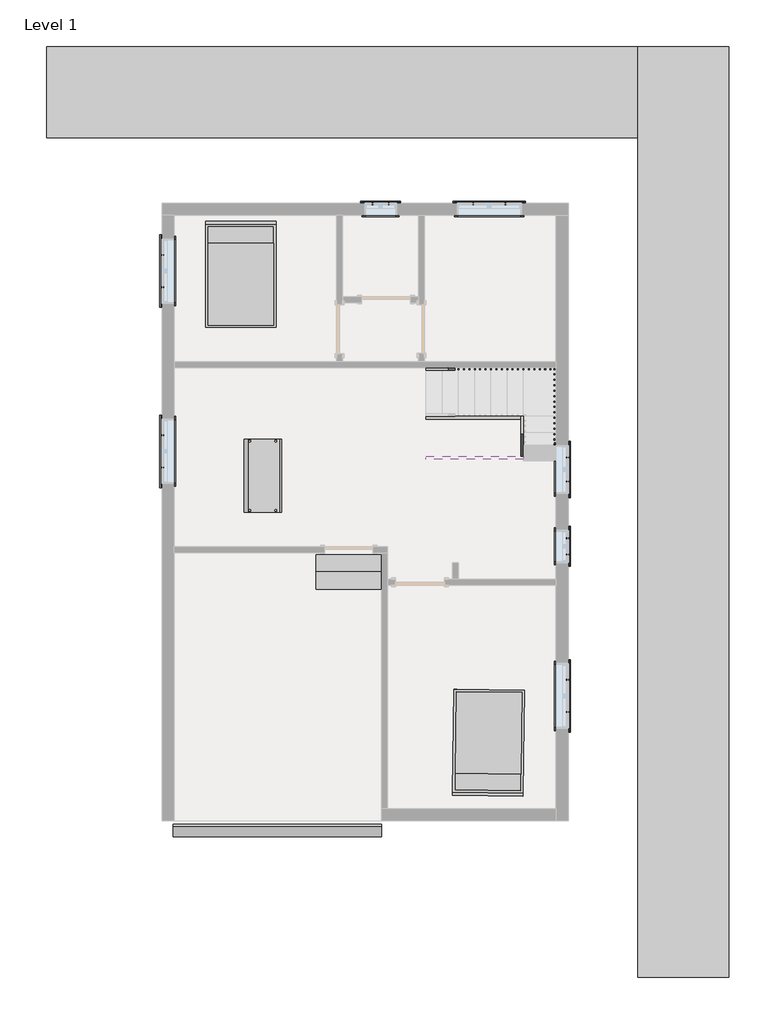
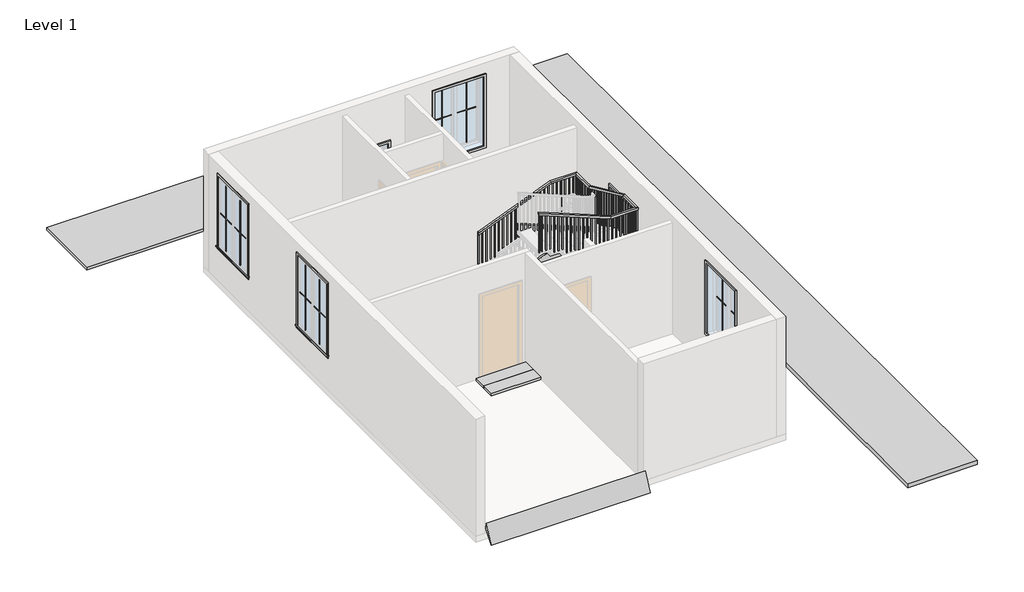
# One storey, part 2 of 2: 33 proxies, 3 members, 2 furniture elements, 1 railing.
"""IFC4 building model written with IfcOpenShell, lengths in millimetres."""

from ifc_helpers import new_model, si_unit, frame, origin, place, context, project, spatial, polyline, outline, extrude, faceted_brep, transform, mapped, element, save
from components import extrusion_extrusion_7330b34c, generic_models_1_generic_models_1_3256bdb4, generic_models_2_generic_models_2_0ca87cec, generic_models_3_generic_models_3_c0206aab, modern_coffee_table_17989_modern_coffee_table_17989_d3a860c8, muntin_pattern_2x2_muntin_pattern_2x2_2b4d9f72, muntin_pattern_2x2_muntin_pattern_2x2_ef995ed3, muntin_pattern_2x2_muntin_pattern_2x2_53152e2c, muntin_pattern_2x2_muntin_pattern_2x2_e8f3e573, muntin_pattern_2x2_muntin_pattern_2x2_9b64c8d5, muntin_pattern_2x2_muntin_pattern_2x2_d319fd2e, trim_window_exterior_flat_with_sill_b7e4d11c, trim_window_exterior_flat_with_sill_a665a915, trim_window_exterior_flat_with_sill_66148908, trim_window_interior_flat_picture_frame_936b8d2a, trim_window_interior_flat_picture_frame_d485c387, trim_window_interior_flat_picture_frame_d5b7f3a4, bed_17739_bed_17739_15c61121

model = new_model("IFC4")

# Units and contexts
model_context = context("Model", 3, world=origin())
ifc_project = project(units=[si_unit("LENGTHUNIT", "METRE", prefix="MILLI")], contexts=[model_context])

# Site, building, storey
site = spatial("IfcSite", under=ifc_project)
building = spatial("IfcBuilding", under=site)
storey = spatial("IfcBuildingStorey", under=building, Name="Level 1", Elevation=0.0)

# Proxies
placement = place(None, origin())
extrusion_extrusion_shape = extrusion_extrusion_7330b34c(model_context)
element("IfcBuildingElementProxy", 1, Name="EXTRUSION : EXTRUSION", ObjectType="EXTRUSION : EXTRUSION", at=placement, inside=storey, context=model_context, shape_type="MappedRepresentation", body=[
    mapped(extrusion_extrusion_shape, transform((0.0, 0.0, 0.0), x_axis=(1.0, 0.0, 0.0), y_axis=(0.0, 1.0, 0.0), z_axis=(0.0, 0.0, 1.0))),
])
generic_models_1_generic_models_1_shape = generic_models_1_generic_models_1_3256bdb4(model_context)
element("IfcBuildingElementProxy", 2, Name="Generic Models 1 : Generic Models 1", ObjectType="Generic Models 1 : Generic Models 1", at=placement, inside=storey, context=model_context, shape_type="MappedRepresentation", body=[
    mapped(generic_models_1_generic_models_1_shape, transform((0.0, 0.0, 0.0), x_axis=(1.0, 0.0, 0.0), y_axis=(0.0, 1.0, 0.0), z_axis=(0.0, 0.0, 1.0))),
])
generic_models_2_generic_models_2_shape = generic_models_2_generic_models_2_0ca87cec(model_context)
element("IfcBuildingElementProxy", 3, Name="Generic Models 2 : Generic Models 2", ObjectType="Generic Models 2 : Generic Models 2", at=placement, inside=storey, context=model_context, shape_type="MappedRepresentation", body=[
    mapped(generic_models_2_generic_models_2_shape, transform((0.0, 0.0, 0.0), x_axis=(1.0, 0.0, 0.0), y_axis=(0.0, 1.0, 0.0), z_axis=(0.0, 0.0, 1.0))),
])
generic_models_3_generic_models_3_shape = generic_models_3_generic_models_3_c0206aab(model_context)
element("IfcBuildingElementProxy", 4, Name="Generic Models 3 : Generic Models 3", ObjectType="Generic Models 3 : Generic Models 3", at=placement, inside=storey, context=model_context, shape_type="MappedRepresentation", body=[
    mapped(generic_models_3_generic_models_3_shape, transform((0.0, 0.0, 0.0), x_axis=(1.0, 0.0, 0.0), y_axis=(0.0, 1.0, 0.0), z_axis=(0.0, 0.0, 1.0))),
])
modern_coffee_table_17989_modern_coffee_table_17989_shape = modern_coffee_table_17989_modern_coffee_table_17989_d3a860c8(model_context)
element("IfcBuildingElementProxy", 5, Name="Modern_Coffee_Table_17989 : Modern_Coffee_Table_17989", ObjectType="Modern_Coffee_Table_17989 : Modern_Coffee_Table_17989", at=placement, inside=storey, context=model_context, shape_type="MappedRepresentation", body=[
    mapped(modern_coffee_table_17989_modern_coffee_table_17989_shape, transform((3060.7, 9172.1823212, 0.0), x_axis=(0.0, 1.0, 0.0), y_axis=(-1.0, 0.0, 0.0), z_axis=(0.0, 0.0, 1.0))),
])
muntin_pattern_2x2_muntin_pattern_2x2_shape = muntin_pattern_2x2_muntin_pattern_2x2_2b4d9f72(model_context)
element("IfcBuildingElementProxy", 6, Name="Muntin Pattern_2x2 : Muntin Pattern_2x2", ObjectType="Muntin Pattern_2x2 : Muntin Pattern_2x2", at=placement, inside=storey, context=model_context, shape_type="MappedRepresentation", body=[
    mapped(muntin_pattern_2x2_muntin_pattern_2x2_shape, transform((1533.525, 12477.4069306, 984.25), x_axis=(0.0, 1.0, 0.0), y_axis=(-1.0, 0.0, 0.0), z_axis=(0.0, 0.0, 1.0))),
])
element("IfcBuildingElementProxy", 7, Name="Muntin Pattern_2x2 : Muntin Pattern_2x2", ObjectType="Muntin Pattern_2x2 : Muntin Pattern_2x2", at=placement, inside=storey, context=model_context, shape_type="MappedRepresentation", body=[
    mapped(muntin_pattern_2x2_muntin_pattern_2x2_shape, transform((7361.2375, 14045.8073212, 984.25), x_axis=(1.0, 0.0, 0.0), y_axis=(0.0, 1.0, 0.0), z_axis=(0.0, 0.0, 1.0))),
])
element("IfcBuildingElementProxy", 8, Name="Muntin Pattern_2x2 : Muntin Pattern_2x2", ObjectType="Muntin Pattern_2x2 : Muntin Pattern_2x2", at=placement, inside=storey, context=model_context, shape_type="MappedRepresentation", body=[
    mapped(muntin_pattern_2x2_muntin_pattern_2x2_shape, transform((9134.475, 5119.2948212, 984.25), x_axis=(0.0, -1.0, 0.0), y_axis=(1.0, 0.0, 0.0), z_axis=(0.0, 0.0, 1.0))),
])
element("IfcBuildingElementProxy", 9, Name="Muntin Pattern_2x2 : Muntin Pattern_2x2", ObjectType="Muntin Pattern_2x2 : Muntin Pattern_2x2", at=placement, inside=storey, context=model_context, shape_type="MappedRepresentation", body=[
    mapped(muntin_pattern_2x2_muntin_pattern_2x2_shape, transform((1533.525, 9097.5698212, 984.25), x_axis=(0.0, 1.0, 0.0), y_axis=(-1.0, 0.0, 0.0), z_axis=(0.0, 0.0, 1.0))),
])
muntin_pattern_2x2_muntin_pattern_2x2_2_shape = muntin_pattern_2x2_muntin_pattern_2x2_ef995ed3(model_context)
element("IfcBuildingElementProxy", 10, Name="Muntin Pattern_2x2 : Muntin Pattern_2x2", ObjectType="Muntin Pattern_2x2 : Muntin Pattern_2x2", at=placement, inside=storey, context=model_context, shape_type="MappedRepresentation", body=[
    mapped(muntin_pattern_2x2_muntin_pattern_2x2_2_shape, transform((1533.525, 13083.8319306, 984.25), x_axis=(0.0, -1.0, 0.0), y_axis=(1.0, 0.0, 0.0), z_axis=(0.0, 0.0, 1.0))),
])
element("IfcBuildingElementProxy", 11, Name="Muntin Pattern_2x2 : Muntin Pattern_2x2", ObjectType="Muntin Pattern_2x2 : Muntin Pattern_2x2", at=placement, inside=storey, context=model_context, shape_type="MappedRepresentation", body=[
    mapped(muntin_pattern_2x2_muntin_pattern_2x2_2_shape, transform((7967.6625, 14045.8073212, 984.25), x_axis=(-1.0, 0.0, 0.0), y_axis=(0.0, -1.0, 0.0), z_axis=(0.0, 0.0, 1.0))),
])
element("IfcBuildingElementProxy", 12, Name="Muntin Pattern_2x2 : Muntin Pattern_2x2", ObjectType="Muntin Pattern_2x2 : Muntin Pattern_2x2", at=placement, inside=storey, context=model_context, shape_type="MappedRepresentation", body=[
    mapped(muntin_pattern_2x2_muntin_pattern_2x2_2_shape, transform((9134.475, 4512.8698212, 984.25), x_axis=(0.0, 1.0, 0.0), y_axis=(-1.0, 0.0, 0.0), z_axis=(0.0, 0.0, 1.0))),
])
element("IfcBuildingElementProxy", 13, Name="Muntin Pattern_2x2 : Muntin Pattern_2x2", ObjectType="Muntin Pattern_2x2 : Muntin Pattern_2x2", at=placement, inside=storey, context=model_context, shape_type="MappedRepresentation", body=[
    mapped(muntin_pattern_2x2_muntin_pattern_2x2_2_shape, transform((1533.525, 9703.9948212, 984.25), x_axis=(0.0, -1.0, 0.0), y_axis=(1.0, 0.0, 0.0), z_axis=(0.0, 0.0, 1.0))),
])
muntin_pattern_2x2_muntin_pattern_2x2_3_shape = muntin_pattern_2x2_muntin_pattern_2x2_53152e2c(model_context)
element("IfcBuildingElementProxy", 14, Name="Muntin Pattern_2x2 : Muntin Pattern_2x2", ObjectType="Muntin Pattern_2x2 : Muntin Pattern_2x2", at=placement, inside=storey, context=model_context, shape_type="MappedRepresentation", body=[
    mapped(muntin_pattern_2x2_muntin_pattern_2x2_3_shape, transform((9134.475, 7771.2135712, 984.25), x_axis=(0.0, -1.0, 0.0), y_axis=(1.0, 0.0, 0.0), z_axis=(0.0, 0.0, 1.0))),
])
element("IfcBuildingElementProxy", 15, Name="Muntin Pattern_2x2 : Muntin Pattern_2x2", ObjectType="Muntin Pattern_2x2 : Muntin Pattern_2x2", at=placement, inside=storey, context=model_context, shape_type="MappedRepresentation", body=[
    mapped(muntin_pattern_2x2_muntin_pattern_2x2_3_shape, transform((5475.2875, 14045.8073212, 984.25), x_axis=(1.0, 0.0, 0.0), y_axis=(0.0, 1.0, 0.0), z_axis=(0.0, 0.0, 1.0))),
])
muntin_pattern_2x2_muntin_pattern_2x2_4_shape = muntin_pattern_2x2_muntin_pattern_2x2_e8f3e573(model_context)
element("IfcBuildingElementProxy", 16, Name="Muntin Pattern_2x2 : Muntin Pattern_2x2", ObjectType="Muntin Pattern_2x2 : Muntin Pattern_2x2", at=placement, inside=storey, context=model_context, shape_type="MappedRepresentation", body=[
    mapped(muntin_pattern_2x2_muntin_pattern_2x2_4_shape, transform((9134.475, 7469.5885712, 984.25), x_axis=(0.0, 1.0, 0.0), y_axis=(-1.0, 0.0, 0.0), z_axis=(0.0, 0.0, 1.0))),
])
element("IfcBuildingElementProxy", 17, Name="Muntin Pattern_2x2 : Muntin Pattern_2x2", ObjectType="Muntin Pattern_2x2 : Muntin Pattern_2x2", at=placement, inside=storey, context=model_context, shape_type="MappedRepresentation", body=[
    mapped(muntin_pattern_2x2_muntin_pattern_2x2_4_shape, transform((5776.9125, 14045.8073212, 984.25), x_axis=(-1.0, 0.0, 0.0), y_axis=(0.0, -1.0, 0.0), z_axis=(0.0, 0.0, 1.0))),
])
muntin_pattern_2x2_muntin_pattern_2x2_5_shape = muntin_pattern_2x2_muntin_pattern_2x2_9b64c8d5(model_context)
element("IfcBuildingElementProxy", 18, Name="Muntin Pattern_2x2 : Muntin Pattern_2x2", ObjectType="Muntin Pattern_2x2 : Muntin Pattern_2x2", at=placement, inside=storey, context=model_context, shape_type="MappedRepresentation", body=[
    mapped(muntin_pattern_2x2_muntin_pattern_2x2_5_shape, transform((9134.475, 9287.1024384, 984.25), x_axis=(0.0, -1.0, 0.0), y_axis=(1.0, 0.0, 0.0), z_axis=(0.0, 0.0, 1.0))),
])
muntin_pattern_2x2_muntin_pattern_2x2_6_shape = muntin_pattern_2x2_muntin_pattern_2x2_d319fd2e(model_context)
element("IfcBuildingElementProxy", 19, Name="Muntin Pattern_2x2 : Muntin Pattern_2x2", ObjectType="Muntin Pattern_2x2 : Muntin Pattern_2x2", at=placement, inside=storey, context=model_context, shape_type="MappedRepresentation", body=[
    mapped(muntin_pattern_2x2_muntin_pattern_2x2_6_shape, transform((9134.475, 8833.0774384, 984.25), x_axis=(0.0, 1.0, 0.0), y_axis=(-1.0, 0.0, 0.0), z_axis=(0.0, 0.0, 1.0))),
])
trim_window_exterior_flat_with_sill_shape = trim_window_exterior_flat_with_sill_b7e4d11c(model_context)
element("IfcBuildingElementProxy", 20, Name="Trim-Window-Exterior-Flat : with Sill", ObjectType="Trim-Window-Exterior-Flat : with Sill", at=placement, inside=storey, context=model_context, shape_type="MappedRepresentation", body=[
    mapped(trim_window_exterior_flat_with_sill_shape, transform((1524.0, 12780.6194306, 2743.2), x_axis=(0.0, -1.0, 0.0), y_axis=(0.0, 0.0, 1.0), z_axis=(-1.0, 0.0, 0.0))),
])
element("IfcBuildingElementProxy", 21, Name="Trim-Window-Exterior-Flat : with Sill", ObjectType="Trim-Window-Exterior-Flat : with Sill", at=placement, inside=storey, context=model_context, shape_type="MappedRepresentation", body=[
    mapped(trim_window_exterior_flat_with_sill_shape, transform((7664.45, 14055.3323212, 2743.2), x_axis=(-1.0, 0.0, 0.0), y_axis=(0.0, 0.0, 1.0), z_axis=(0.0, 1.0, 0.0))),
])
element("IfcBuildingElementProxy", 22, Name="Trim-Window-Exterior-Flat : with Sill", ObjectType="Trim-Window-Exterior-Flat : with Sill", at=placement, inside=storey, context=model_context, shape_type="MappedRepresentation", body=[
    mapped(trim_window_exterior_flat_with_sill_shape, transform((9144.0, 4816.0823212, 2743.2), x_axis=(0.0, 1.0, 0.0), y_axis=(0.0, 0.0, 1.0), z_axis=(1.0, 0.0, 0.0))),
])
element("IfcBuildingElementProxy", 23, Name="Trim-Window-Exterior-Flat : with Sill", ObjectType="Trim-Window-Exterior-Flat : with Sill", at=placement, inside=storey, context=model_context, shape_type="MappedRepresentation", body=[
    mapped(trim_window_exterior_flat_with_sill_shape, transform((1524.0, 9400.7823212, 2743.2), x_axis=(0.0, -1.0, 0.0), y_axis=(0.0, 0.0, 1.0), z_axis=(-1.0, 0.0, 0.0))),
])
trim_window_exterior_flat_with_sill_2_shape = trim_window_exterior_flat_with_sill_a665a915(model_context)
element("IfcBuildingElementProxy", 24, Name="Trim-Window-Exterior-Flat : with Sill", ObjectType="Trim-Window-Exterior-Flat : with Sill", at=placement, inside=storey, context=model_context, shape_type="MappedRepresentation", body=[
    mapped(trim_window_exterior_flat_with_sill_2_shape, transform((9144.0, 7620.4010712, 1828.8), x_axis=(0.0, 1.0, 0.0), y_axis=(0.0, 0.0, 1.0), z_axis=(1.0, 0.0, 0.0))),
])
element("IfcBuildingElementProxy", 25, Name="Trim-Window-Exterior-Flat : with Sill", ObjectType="Trim-Window-Exterior-Flat : with Sill", at=placement, inside=storey, context=model_context, shape_type="MappedRepresentation", body=[
    mapped(trim_window_exterior_flat_with_sill_2_shape, transform((5626.1, 14055.3323212, 1828.8), x_axis=(-1.0, 0.0, 0.0), y_axis=(0.0, 0.0, 1.0), z_axis=(0.0, 1.0, 0.0))),
])
trim_window_exterior_flat_with_sill_3_shape = trim_window_exterior_flat_with_sill_66148908(model_context)
element("IfcBuildingElementProxy", 26, Name="Trim-Window-Exterior-Flat : with Sill", ObjectType="Trim-Window-Exterior-Flat : with Sill", at=placement, inside=storey, context=model_context, shape_type="MappedRepresentation", body=[
    mapped(trim_window_exterior_flat_with_sill_3_shape, transform((9144.0, 9060.0899384, 2260.6), x_axis=(0.0, 1.0, 0.0), y_axis=(0.0, 0.0, 1.0), z_axis=(1.0, 0.0, 0.0))),
])
trim_window_interior_flat_picture_frame_shape = trim_window_interior_flat_picture_frame_936b8d2a(model_context)
element("IfcBuildingElementProxy", 27, Name="Trim-Window-Interior-Flat : Picture Frame", ObjectType="Trim-Window-Interior-Flat : Picture Frame", at=placement, inside=storey, context=model_context, shape_type="MappedRepresentation", body=[
    mapped(trim_window_interior_flat_picture_frame_shape, transform((1752.6, 12780.6194306, 2743.2), x_axis=(0.0, 1.0, 0.0), y_axis=(0.0, 0.0, 1.0), z_axis=(1.0, 0.0, 0.0))),
])
element("IfcBuildingElementProxy", 28, Name="Trim-Window-Interior-Flat : Picture Frame", ObjectType="Trim-Window-Interior-Flat : Picture Frame", at=placement, inside=storey, context=model_context, shape_type="MappedRepresentation", body=[
    mapped(trim_window_interior_flat_picture_frame_shape, transform((7664.45, 13826.7323212, 2743.2), x_axis=(1.0, 0.0, 0.0), y_axis=(0.0, 0.0, 1.0), z_axis=(0.0, -1.0, 0.0))),
])
element("IfcBuildingElementProxy", 29, Name="Trim-Window-Interior-Flat : Picture Frame", ObjectType="Trim-Window-Interior-Flat : Picture Frame", at=placement, inside=storey, context=model_context, shape_type="MappedRepresentation", body=[
    mapped(trim_window_interior_flat_picture_frame_shape, transform((8915.4, 4816.0823212, 2743.2), x_axis=(0.0, -1.0, 0.0), y_axis=(0.0, 0.0, 1.0), z_axis=(-1.0, 0.0, 0.0))),
])
element("IfcBuildingElementProxy", 30, Name="Trim-Window-Interior-Flat : Picture Frame", ObjectType="Trim-Window-Interior-Flat : Picture Frame", at=placement, inside=storey, context=model_context, shape_type="MappedRepresentation", body=[
    mapped(trim_window_interior_flat_picture_frame_shape, transform((1752.6, 9400.7823212, 2743.2), x_axis=(0.0, 1.0, 0.0), y_axis=(0.0, 0.0, 1.0), z_axis=(1.0, 0.0, 0.0))),
])
trim_window_interior_flat_picture_frame_2_shape = trim_window_interior_flat_picture_frame_d485c387(model_context)
element("IfcBuildingElementProxy", 31, Name="Trim-Window-Interior-Flat : Picture Frame", ObjectType="Trim-Window-Interior-Flat : Picture Frame", at=placement, inside=storey, context=model_context, shape_type="MappedRepresentation", body=[
    mapped(trim_window_interior_flat_picture_frame_2_shape, transform((8915.4, 7620.4010712, 1828.8), x_axis=(0.0, -1.0, 0.0), y_axis=(0.0, 0.0, 1.0), z_axis=(-1.0, 0.0, 0.0))),
])
element("IfcBuildingElementProxy", 32, Name="Trim-Window-Interior-Flat : Picture Frame", ObjectType="Trim-Window-Interior-Flat : Picture Frame", at=placement, inside=storey, context=model_context, shape_type="MappedRepresentation", body=[
    mapped(trim_window_interior_flat_picture_frame_2_shape, transform((5626.1, 13826.7323212, 1828.8), x_axis=(1.0, 0.0, 0.0), y_axis=(0.0, 0.0, 1.0), z_axis=(0.0, -1.0, 0.0))),
])
trim_window_interior_flat_picture_frame_3_shape = trim_window_interior_flat_picture_frame_d5b7f3a4(model_context)
element("IfcBuildingElementProxy", 33, Name="Trim-Window-Interior-Flat : Picture Frame", ObjectType="Trim-Window-Interior-Flat : Picture Frame", at=placement, inside=storey, context=model_context, shape_type="MappedRepresentation", body=[
    mapped(trim_window_interior_flat_picture_frame_3_shape, transform((8915.4, 9060.0899384, 2260.6), x_axis=(0.0, -1.0, 0.0), y_axis=(0.0, 0.0, 1.0), z_axis=(-1.0, 0.0, 0.0))),
])

# Furniture
bed_17739_bed_17739_shape = bed_17739_bed_17739_15c61121(model_context)
element("IfcFurniture", 34, ObjectType="Bed_17739 : Bed_17739", at=placement, inside=storey, context=model_context, shape_type="MappedRepresentation", body=[
    mapped(bed_17739_bed_17739_shape, transform((3003.55, 12696.4323212, 0.0), x_axis=(1.0, 0.0, 0.0), y_axis=(0.0, 1.0, 0.0), z_axis=(0.0, 0.0, 1.0))),
])
element("IfcFurniture", 35, ObjectType="Bed_17739 : Bed_17739", at=placement, inside=storey, context=model_context, shape_type="MappedRepresentation", body=[
    mapped(bed_17739_bed_17739_shape, transform((7650.1504891, 3963.5673274, 0.0), x_axis=(-0.9999063358908578, 0.013686469424921632, 0.0), y_axis=(-0.013686469424921632, -0.9999063358908578, 0.0), z_axis=(0.0, 0.0, 1.0))),
])

# Members
element("IfcMember", 36, ObjectType="Stringer - 2\" Width", at=placement, inside=storey, context=model_context, shape_type="SweptSolid", body=[
    extrude(outline(polyline([(196.3880536, 6477.0), (0.0, 6477.0), (0.0, 6806.7289826), (579.3084069, 8255.0), (907.5880536, 8255.0), (196.3880536, 6477.0)])), frame((0.0, 10004.0323212, 0.0), z_axis=(0.0, 1.0, 0.0), x_axis=(0.0, 0.0, 1.0)), (0.0, 0.0, 1.0), 50.8),
])
element("IfcMember", 37, ObjectType="Stringer - 2\" Width", at=placement, inside=storey, context=model_context, shape_type="SweptSolid", body=[
    extrude(outline(polyline([(10054.8323212, 1053.4437705), (10054.8323212, 718.3051732), (9305.5323212, 1060.842316), (9305.5323212, 1395.9809133), (10054.8323212, 1053.4437705)])), frame((8255.0, 0.0, 0.0), z_axis=(1.0, 0.0, 0.0), x_axis=(0.0, 1.0, 0.0)), (0.0, 0.0, 1.0), 50.8),
])
element("IfcMember", 38, ObjectType="Stringer - 2\" Width", at=placement, inside=storey, context=model_context, shape_type="SweptSolid", body=[
    extrude(outline(polyline([(1209.2284069, 8305.8), (1537.5080536, 8305.8), (2269.0280536, 6477.0), (1940.7484069, 6477.0), (1209.2284069, 8305.8)])), frame((0.0, 9254.7323212, 0.0), z_axis=(0.0, 1.0, 0.0), x_axis=(0.0, 0.0, 1.0)), (0.0, 0.0, 1.0), 50.8),
])

# Railing
element("IfcRailing", 39, ObjectType="Handrail - Rectangular", at=placement, inside=storey, context=model_context, shape_type="SolidModel", body=[
    faceted_brep([(6477.0, 10969.2323212, 1036.32), (6477.0, 10969.2323212, 981.6067256), (6477.0, 10918.4323212, 981.6067256), (6477.0, 10918.4323212, 1036.32), (8242.3, 10969.2323212, 1742.44), (8252.0831861, 10969.2323212, 1691.64), (8252.0831861, 10918.4323212, 1691.64), (8242.3, 10918.4323212, 1742.44), (8915.4, 10969.2323212, 1742.44), (8915.4, 10969.2323212, 1691.64), (8864.6, 10918.4323212, 1691.64), (8864.6, 10918.4323212, 1742.44), (8915.4, 10377.0948212, 1742.44), (8915.4, 10366.0338743, 1691.64), (8864.6, 10366.0338743, 1691.64), (8864.6, 10377.0948212, 1742.44), (8915.4, 8932.4698212, 2402.84), (8915.4, 8921.4088743, 2352.04), (8864.6, 8921.4088743, 2352.04), (8864.6, 8932.4698212, 2402.84), (8915.4, 8340.3323212, 2402.84), (8915.4, 8340.3323212, 2352.04), (8864.6, 8391.1323212, 2352.04), (8864.6, 8391.1323212, 2402.84), (8242.3, 8340.3323212, 2402.84), (8232.5168139, 8340.3323212, 2352.04), (8232.5168139, 8391.1323212, 2352.04), (8242.3, 8391.1323212, 2402.84), (6477.0, 8340.3323212, 3108.96), (6477.0, 8391.1323212, 3108.96), (6477.0, 8391.1323212, 3054.2467256), (6477.0, 8340.3323212, 3054.2467256)], [[[0, 1, 2, 3]], [[1, 0, 4, 5]], [[2, 1, 5, 6]], [[3, 2, 6, 7]], [[0, 3, 7, 4]], [[5, 4, 8, 9]], [[6, 5, 9, 10]], [[7, 6, 10, 11]], [[4, 7, 11, 8]], [[9, 8, 12, 13]], [[10, 9, 13, 14]], [[11, 10, 14, 15]], [[8, 11, 15, 12]], [[13, 12, 16, 17]], [[14, 13, 17, 18]], [[15, 14, 18, 19]], [[12, 15, 19, 16]], [[17, 16, 20, 21]], [[18, 17, 21, 22]], [[19, 18, 22, 23]], [[16, 19, 23, 20]], [[21, 20, 24, 25]], [[22, 21, 25, 26]], [[23, 22, 26, 27]], [[20, 23, 27, 24]], [[28, 29, 30, 31]], [[25, 24, 28, 31]], [[26, 25, 31, 30]], [[27, 26, 30, 29]], [[24, 27, 29, 28]]]),
    extrude(outline(polyline([(3027.5767256, 6543.675), (2072.64, 6543.675), (2072.64, 6562.725), (3019.9567256, 6562.725), (3027.5767256, 6543.675)])), frame((0.0, 8356.2073212, 0.0), z_axis=(0.0, 1.0, 0.0), x_axis=(0.0, 0.0, 1.0)), (0.0, 0.0, 1.0), 19.05),
    extrude(outline(polyline([(2986.9367256, 6645.275), (2072.64, 6645.275), (2072.64, 6664.325), (2979.3167256, 6664.325), (2986.9367256, 6645.275)])), frame((0.0, 8356.2073212, 0.0), z_axis=(0.0, 1.0, 0.0), x_axis=(0.0, 0.0, 1.0)), (0.0, 0.0, 1.0), 19.05),
    extrude(outline(polyline([(2946.2967256, 6746.875), (2072.64, 6746.875), (2072.64, 6765.925), (2938.6767256, 6765.925), (2946.2967256, 6746.875)])), frame((0.0, 8356.2073212, 0.0), z_axis=(0.0, 1.0, 0.0), x_axis=(0.0, 0.0, 1.0)), (0.0, 0.0, 1.0), 19.05),
    extrude(outline(polyline([(2905.6567256, 6848.475), (1950.72, 6848.475), (1950.72, 6867.525), (2898.0367256, 6867.525), (2905.6567256, 6848.475)])), frame((0.0, 8356.2073212, 0.0), z_axis=(0.0, 1.0, 0.0), x_axis=(0.0, 0.0, 1.0)), (0.0, 0.0, 1.0), 19.05),
    extrude(outline(polyline([(2865.0167256, 6950.075), (1950.72, 6950.075), (1950.72, 6969.125), (2857.3967256, 6969.125), (2865.0167256, 6950.075)])), frame((0.0, 8356.2073212, 0.0), z_axis=(0.0, 1.0, 0.0), x_axis=(0.0, 0.0, 1.0)), (0.0, 0.0, 1.0), 19.05),
    extrude(outline(polyline([(2824.3767256, 7051.675), (1950.72, 7051.675), (1950.72, 7070.725), (2816.7567256, 7070.725), (2824.3767256, 7051.675)])), frame((0.0, 8356.2073212, 0.0), z_axis=(0.0, 1.0, 0.0), x_axis=(0.0, 0.0, 1.0)), (0.0, 0.0, 1.0), 19.05),
    extrude(outline(polyline([(2783.7367256, 7153.275), (1828.8, 7153.275), (1828.8, 7172.325), (2776.1167256, 7172.325), (2783.7367256, 7153.275)])), frame((0.0, 8356.2073212, 0.0), z_axis=(0.0, 1.0, 0.0), x_axis=(0.0, 0.0, 1.0)), (0.0, 0.0, 1.0), 19.05),
    extrude(outline(polyline([(2743.0967256, 7254.875), (1828.8, 7254.875), (1828.8, 7273.925), (2735.4767256, 7273.925), (2743.0967256, 7254.875)])), frame((0.0, 8356.2073212, 0.0), z_axis=(0.0, 1.0, 0.0), x_axis=(0.0, 0.0, 1.0)), (0.0, 0.0, 1.0), 19.05),
    extrude(outline(polyline([(2702.4567256, 7356.475), (1828.8, 7356.475), (1828.8, 7375.525), (2694.8367256, 7375.525), (2702.4567256, 7356.475)])), frame((0.0, 8356.2073212, 0.0), z_axis=(0.0, 1.0, 0.0), x_axis=(0.0, 0.0, 1.0)), (0.0, 0.0, 1.0), 19.05),
    extrude(outline(polyline([(2661.8167256, 7458.075), (1706.88, 7458.075), (1706.88, 7477.125), (2654.1967256, 7477.125), (2661.8167256, 7458.075)])), frame((0.0, 8356.2073212, 0.0), z_axis=(0.0, 1.0, 0.0), x_axis=(0.0, 0.0, 1.0)), (0.0, 0.0, 1.0), 19.05),
    extrude(outline(polyline([(2621.1767256, 7559.675), (1706.88, 7559.675), (1706.88, 7578.725), (2613.5567256, 7578.725), (2621.1767256, 7559.675)])), frame((0.0, 8356.2073212, 0.0), z_axis=(0.0, 1.0, 0.0), x_axis=(0.0, 0.0, 1.0)), (0.0, 0.0, 1.0), 19.05),
    extrude(outline(polyline([(2580.5367256, 7661.275), (1706.88, 7661.275), (1706.88, 7680.325), (2572.9167256, 7680.325), (2580.5367256, 7661.275)])), frame((0.0, 8356.2073212, 0.0), z_axis=(0.0, 1.0, 0.0), x_axis=(0.0, 0.0, 1.0)), (0.0, 0.0, 1.0), 19.05),
    extrude(outline(polyline([(2539.8967256, 7762.875), (1584.96, 7762.875), (1584.96, 7781.925), (2532.2767256, 7781.925), (2539.8967256, 7762.875)])), frame((0.0, 8356.2073212, 0.0), z_axis=(0.0, 1.0, 0.0), x_axis=(0.0, 0.0, 1.0)), (0.0, 0.0, 1.0), 19.05),
    extrude(outline(polyline([(2499.2567256, 7864.475), (1584.96, 7864.475), (1584.96, 7883.525), (2491.6367256, 7883.525), (2499.2567256, 7864.475)])), frame((0.0, 8356.2073212, 0.0), z_axis=(0.0, 1.0, 0.0), x_axis=(0.0, 0.0, 1.0)), (0.0, 0.0, 1.0), 19.05),
    extrude(outline(polyline([(2458.6167256, 7966.075), (1584.96, 7966.075), (1584.96, 7985.125), (2450.9967256, 7985.125), (2458.6167256, 7966.075)])), frame((0.0, 8356.2073212, 0.0), z_axis=(0.0, 1.0, 0.0), x_axis=(0.0, 0.0, 1.0)), (0.0, 0.0, 1.0), 19.05),
    extrude(outline(polyline([(2417.9767256, 8067.675), (1463.04, 8067.675), (1463.04, 8086.725), (2410.3567256, 8086.725), (2417.9767256, 8067.675)])), frame((0.0, 8356.2073212, 0.0), z_axis=(0.0, 1.0, 0.0), x_axis=(0.0, 0.0, 1.0)), (0.0, 0.0, 1.0), 19.05),
    extrude(outline(polyline([(2377.3367256, 8169.275), (1463.04, 8169.275), (1463.04, 8188.325), (2369.7167256, 8188.325), (2377.3367256, 8169.275)])), frame((0.0, 8356.2073212, 0.0), z_axis=(0.0, 1.0, 0.0), x_axis=(0.0, 0.0, 1.0)), (0.0, 0.0, 1.0), 19.05),
    extrude(outline(polyline([(8289.925, 8356.2073212), (8270.875, 8356.2073212), (8270.875, 8375.2573212), (8289.925, 8375.2573212), (8289.925, 8356.2073212)])), frame((0.0, 0.0, 1463.04), z_axis=(0.0, 0.0, 1.0), x_axis=(1.0, 0.0, 0.0)), (0.0, 0.0, 1.0), 889.0),
    extrude(outline(polyline([(8391.525, 8356.2073212), (8372.475, 8356.2073212), (8372.475, 8375.2573212), (8391.525, 8375.2573212), (8391.525, 8356.2073212)])), frame((0.0, 0.0, 1341.12), z_axis=(0.0, 0.0, 1.0), x_axis=(1.0, 0.0, 0.0)), (0.0, 0.0, 1.0), 1010.92),
    extrude(outline(polyline([(8493.125, 8356.2073212), (8474.075, 8356.2073212), (8474.075, 8375.2573212), (8493.125, 8375.2573212), (8493.125, 8356.2073212)])), frame((0.0, 0.0, 1341.12), z_axis=(0.0, 0.0, 1.0), x_axis=(1.0, 0.0, 0.0)), (0.0, 0.0, 1.0), 1010.92),
    extrude(outline(polyline([(8594.725, 8356.2073212), (8575.675, 8356.2073212), (8575.675, 8375.2573212), (8594.725, 8375.2573212), (8594.725, 8356.2073212)])), frame((0.0, 0.0, 1341.12), z_axis=(0.0, 0.0, 1.0), x_axis=(1.0, 0.0, 0.0)), (0.0, 0.0, 1.0), 1010.92),
    extrude(outline(polyline([(8696.325, 8356.2073212), (8677.275, 8356.2073212), (8677.275, 8375.2573212), (8696.325, 8375.2573212), (8696.325, 8356.2073212)])), frame((0.0, 0.0, 1341.12), z_axis=(0.0, 0.0, 1.0), x_axis=(1.0, 0.0, 0.0)), (0.0, 0.0, 1.0), 1010.92),
    extrude(outline(polyline([(8797.925, 8356.2073212), (8778.875, 8356.2073212), (8778.875, 8375.2573212), (8797.925, 8375.2573212), (8797.925, 8356.2073212)])), frame((0.0, 0.0, 1341.12), z_axis=(0.0, 0.0, 1.0), x_axis=(1.0, 0.0, 0.0)), (0.0, 0.0, 1.0), 1010.92),
    extrude(outline(polyline([(8899.525, 8413.3573212), (8899.525, 8394.3073212), (8880.475, 8394.3073212), (8880.475, 8413.3573212), (8899.525, 8413.3573212)])), frame((0.0, 0.0, 1341.12), z_axis=(0.0, 0.0, 1.0), x_axis=(1.0, 0.0, 0.0)), (0.0, 0.0, 1.0), 1010.92),
    extrude(outline(polyline([(8899.525, 8514.9573212), (8899.525, 8495.9073212), (8880.475, 8495.9073212), (8880.475, 8514.9573212), (8899.525, 8514.9573212)])), frame((0.0, 0.0, 1341.12), z_axis=(0.0, 0.0, 1.0), x_axis=(1.0, 0.0, 0.0)), (0.0, 0.0, 1.0), 1010.92),
    extrude(outline(polyline([(8899.525, 8616.5573212), (8899.525, 8597.5073212), (8880.475, 8597.5073212), (8880.475, 8616.5573212), (8899.525, 8616.5573212)])), frame((0.0, 0.0, 1341.12), z_axis=(0.0, 0.0, 1.0), x_axis=(1.0, 0.0, 0.0)), (0.0, 0.0, 1.0), 1010.92),
    extrude(outline(polyline([(8899.525, 8718.1573212), (8899.525, 8699.1073212), (8880.475, 8699.1073212), (8880.475, 8718.1573212), (8899.525, 8718.1573212)])), frame((0.0, 0.0, 1341.12), z_axis=(0.0, 0.0, 1.0), x_axis=(1.0, 0.0, 0.0)), (0.0, 0.0, 1.0), 1010.92),
    extrude(outline(polyline([(8899.525, 8819.7573212), (8899.525, 8800.7073212), (8880.475, 8800.7073212), (8880.475, 8819.7573212), (8899.525, 8819.7573212)])), frame((0.0, 0.0, 1341.12), z_axis=(0.0, 0.0, 1.0), x_axis=(1.0, 0.0, 0.0)), (0.0, 0.0, 1.0), 1010.92),
    extrude(outline(polyline([(8899.525, 8921.3573212), (8899.525, 8902.3073212), (8880.475, 8902.3073212), (8880.475, 8921.3573212), (8899.525, 8921.3573212)])), frame((0.0, 0.0, 1341.12), z_axis=(0.0, 0.0, 1.0), x_axis=(1.0, 0.0, 0.0)), (0.0, 0.0, 1.0), 1010.92),
    extrude(outline(polyline([(9022.9573212, 2305.6178528), (9022.9573212, 1341.12), (9003.9073212, 1341.12), (9003.9073212, 2314.3264243), (9022.9573212, 2305.6178528)])), frame((8880.475, 0.0, 0.0), z_axis=(1.0, 0.0, 0.0), x_axis=(0.0, 1.0, 0.0)), (0.0, 0.0, 1.0), 19.05),
    extrude(outline(polyline([(9124.5573212, 2259.1721386), (9124.5573212, 1341.12), (9105.5073212, 1341.12), (9105.5073212, 2267.88071), (9124.5573212, 2259.1721386)])), frame((8880.475, 0.0, 0.0), z_axis=(1.0, 0.0, 0.0), x_axis=(0.0, 1.0, 0.0)), (0.0, 0.0, 1.0), 19.05),
    extrude(outline(polyline([(9226.1573212, 2212.7264243), (9226.1573212, 1341.12), (9207.1073212, 1341.12), (9207.1073212, 2221.4349957), (9226.1573212, 2212.7264243)])), frame((8880.475, 0.0, 0.0), z_axis=(1.0, 0.0, 0.0), x_axis=(0.0, 1.0, 0.0)), (0.0, 0.0, 1.0), 19.05),
    extrude(outline(polyline([(9327.7573212, 2166.28071), (9327.7573212, 1219.2), (9308.7073212, 1219.2), (9308.7073212, 2174.9892814), (9327.7573212, 2166.28071)])), frame((8880.475, 0.0, 0.0), z_axis=(1.0, 0.0, 0.0), x_axis=(0.0, 1.0, 0.0)), (0.0, 0.0, 1.0), 19.05),
    extrude(outline(polyline([(9429.3573212, 2119.8349957), (9429.3573212, 1219.2), (9410.3073212, 1219.2), (9410.3073212, 2128.5435671), (9429.3573212, 2119.8349957)])), frame((8880.475, 0.0, 0.0), z_axis=(1.0, 0.0, 0.0), x_axis=(0.0, 1.0, 0.0)), (0.0, 0.0, 1.0), 19.05),
    extrude(outline(polyline([(9530.9573212, 2073.3892814), (9530.9573212, 1097.28), (9511.9073212, 1097.28), (9511.9073212, 2082.0978528), (9530.9573212, 2073.3892814)])), frame((8880.475, 0.0, 0.0), z_axis=(1.0, 0.0, 0.0), x_axis=(0.0, 1.0, 0.0)), (0.0, 0.0, 1.0), 19.05),
    extrude(outline(polyline([(9632.5573212, 2026.9435671), (9632.5573212, 1097.28), (9613.5073212, 1097.28), (9613.5073212, 2035.6521386), (9632.5573212, 2026.9435671)])), frame((8880.475, 0.0, 0.0), z_axis=(1.0, 0.0, 0.0), x_axis=(0.0, 1.0, 0.0)), (0.0, 0.0, 1.0), 19.05),
    extrude(outline(polyline([(9734.1573212, 1980.4978528), (9734.1573212, 1097.28), (9715.1073212, 1097.28), (9715.1073212, 1989.2064243), (9734.1573212, 1980.4978528)])), frame((8880.475, 0.0, 0.0), z_axis=(1.0, 0.0, 0.0), x_axis=(0.0, 1.0, 0.0)), (0.0, 0.0, 1.0), 19.05),
    extrude(outline(polyline([(9835.7573212, 1934.0521386), (9835.7573212, 975.36), (9816.7073212, 975.36), (9816.7073212, 1942.76071), (9835.7573212, 1934.0521386)])), frame((8880.475, 0.0, 0.0), z_axis=(1.0, 0.0, 0.0), x_axis=(0.0, 1.0, 0.0)), (0.0, 0.0, 1.0), 19.05),
    extrude(outline(polyline([(9937.3573212, 1887.6064243), (9937.3573212, 975.36), (9918.3073212, 975.36), (9918.3073212, 1896.3149957), (9937.3573212, 1887.6064243)])), frame((8880.475, 0.0, 0.0), z_axis=(1.0, 0.0, 0.0), x_axis=(0.0, 1.0, 0.0)), (0.0, 0.0, 1.0), 19.05),
    extrude(outline(polyline([(10038.9573212, 1841.16071), (10038.9573212, 975.36), (10019.9073212, 975.36), (10019.9073212, 1849.8692814), (10038.9573212, 1841.16071)])), frame((8880.475, 0.0, 0.0), z_axis=(1.0, 0.0, 0.0), x_axis=(0.0, 1.0, 0.0)), (0.0, 0.0, 1.0), 19.05),
    extrude(outline(polyline([(10140.5573212, 1794.7149957), (10140.5573212, 853.44), (10121.5073212, 853.44), (10121.5073212, 1803.4235671), (10140.5573212, 1794.7149957)])), frame((8880.475, 0.0, 0.0), z_axis=(1.0, 0.0, 0.0), x_axis=(0.0, 1.0, 0.0)), (0.0, 0.0, 1.0), 19.05),
    extrude(outline(polyline([(10242.1573212, 1748.2692814), (10242.1573212, 853.44), (10223.1073212, 853.44), (10223.1073212, 1756.9778528), (10242.1573212, 1748.2692814)])), frame((8880.475, 0.0, 0.0), z_axis=(1.0, 0.0, 0.0), x_axis=(0.0, 1.0, 0.0)), (0.0, 0.0, 1.0), 19.05),
    extrude(outline(polyline([(10343.7573212, 1701.8235671), (10343.7573212, 853.44), (10324.7073212, 853.44), (10324.7073212, 1710.5321386), (10343.7573212, 1701.8235671)])), frame((8880.475, 0.0, 0.0), z_axis=(1.0, 0.0, 0.0), x_axis=(0.0, 1.0, 0.0)), (0.0, 0.0, 1.0), 19.05),
    extrude(outline(polyline([(8899.525, 10445.3573212), (8899.525, 10426.3073212), (8880.475, 10426.3073212), (8880.475, 10445.3573212), (8899.525, 10445.3573212)])), frame((0.0, 0.0, 853.44), z_axis=(0.0, 0.0, 1.0), x_axis=(1.0, 0.0, 0.0)), (0.0, 0.0, 1.0), 838.2),
    extrude(outline(polyline([(8899.525, 10546.9573212), (8899.525, 10527.9073212), (8880.475, 10527.9073212), (8880.475, 10546.9573212), (8899.525, 10546.9573212)])), frame((0.0, 0.0, 853.44), z_axis=(0.0, 0.0, 1.0), x_axis=(1.0, 0.0, 0.0)), (0.0, 0.0, 1.0), 838.2),
    extrude(outline(polyline([(8899.525, 10648.5573212), (8899.525, 10629.5073212), (8880.475, 10629.5073212), (8880.475, 10648.5573212), (8899.525, 10648.5573212)])), frame((0.0, 0.0, 853.44), z_axis=(0.0, 0.0, 1.0), x_axis=(1.0, 0.0, 0.0)), (0.0, 0.0, 1.0), 838.2),
    extrude(outline(polyline([(8899.525, 10750.1573212), (8899.525, 10731.1073212), (8880.475, 10731.1073212), (8880.475, 10750.1573212), (8899.525, 10750.1573212)])), frame((0.0, 0.0, 853.44), z_axis=(0.0, 0.0, 1.0), x_axis=(1.0, 0.0, 0.0)), (0.0, 0.0, 1.0), 838.2),
    extrude(outline(polyline([(8899.525, 10851.7573212), (8899.525, 10832.7073212), (8880.475, 10832.7073212), (8880.475, 10851.7573212), (8899.525, 10851.7573212)])), frame((0.0, 0.0, 853.44), z_axis=(0.0, 0.0, 1.0), x_axis=(1.0, 0.0, 0.0)), (0.0, 0.0, 1.0), 838.2),
    extrude(outline(polyline([(8804.275, 10953.3573212), (8823.325, 10953.3573212), (8823.325, 10934.3073212), (8804.275, 10934.3073212), (8804.275, 10953.3573212)])), frame((0.0, 0.0, 853.44), z_axis=(0.0, 0.0, 1.0), x_axis=(1.0, 0.0, 0.0)), (0.0, 0.0, 1.0), 838.2),
    extrude(outline(polyline([(8702.675, 10953.3573212), (8721.725, 10953.3573212), (8721.725, 10934.3073212), (8702.675, 10934.3073212), (8702.675, 10953.3573212)])), frame((0.0, 0.0, 853.44), z_axis=(0.0, 0.0, 1.0), x_axis=(1.0, 0.0, 0.0)), (0.0, 0.0, 1.0), 838.2),
    extrude(outline(polyline([(8601.075, 10953.3573212), (8620.125, 10953.3573212), (8620.125, 10934.3073212), (8601.075, 10934.3073212), (8601.075, 10953.3573212)])), frame((0.0, 0.0, 853.44), z_axis=(0.0, 0.0, 1.0), x_axis=(1.0, 0.0, 0.0)), (0.0, 0.0, 1.0), 838.2),
    extrude(outline(polyline([(8499.475, 10953.3573212), (8518.525, 10953.3573212), (8518.525, 10934.3073212), (8499.475, 10934.3073212), (8499.475, 10953.3573212)])), frame((0.0, 0.0, 853.44), z_axis=(0.0, 0.0, 1.0), x_axis=(1.0, 0.0, 0.0)), (0.0, 0.0, 1.0), 838.2),
    extrude(outline(polyline([(8397.875, 10953.3573212), (8416.925, 10953.3573212), (8416.925, 10934.3073212), (8397.875, 10934.3073212), (8397.875, 10953.3573212)])), frame((0.0, 0.0, 853.44), z_axis=(0.0, 0.0, 1.0), x_axis=(1.0, 0.0, 0.0)), (0.0, 0.0, 1.0), 838.2),
    extrude(outline(polyline([(8296.275, 10953.3573212), (8315.325, 10953.3573212), (8315.325, 10934.3073212), (8296.275, 10934.3073212), (8296.275, 10953.3573212)])), frame((0.0, 0.0, 853.44), z_axis=(0.0, 0.0, 1.0), x_axis=(1.0, 0.0, 0.0)), (0.0, 0.0, 1.0), 838.2),
    extrude(outline(polyline([(1668.6767256, 8194.675), (731.52, 8194.675), (731.52, 8213.725), (1676.2967256, 8213.725), (1668.6767256, 8194.675)])), frame((0.0, 10934.3073212, 0.0), z_axis=(0.0, 1.0, 0.0), x_axis=(0.0, 0.0, 1.0)), (0.0, 0.0, 1.0), 19.05),
    extrude(outline(polyline([(1628.0367256, 8093.075), (731.52, 8093.075), (731.52, 8112.125), (1635.6567256, 8112.125), (1628.0367256, 8093.075)])), frame((0.0, 10934.3073212, 0.0), z_axis=(0.0, 1.0, 0.0), x_axis=(0.0, 0.0, 1.0)), (0.0, 0.0, 1.0), 19.05),
    extrude(outline(polyline([(1587.3967256, 7991.475), (731.52, 7991.475), (731.52, 8010.525), (1595.0167256, 8010.525), (1587.3967256, 7991.475)])), frame((0.0, 10934.3073212, 0.0), z_axis=(0.0, 1.0, 0.0), x_axis=(0.0, 0.0, 1.0)), (0.0, 0.0, 1.0), 19.05),
    extrude(outline(polyline([(1546.7567256, 7889.875), (609.6, 7889.875), (609.6, 7908.925), (1554.3767256, 7908.925), (1546.7567256, 7889.875)])), frame((0.0, 10934.3073212, 0.0), z_axis=(0.0, 1.0, 0.0), x_axis=(0.0, 0.0, 1.0)), (0.0, 0.0, 1.0), 19.05),
    extrude(outline(polyline([(1506.1167256, 7788.275), (609.6, 7788.275), (609.6, 7807.325), (1513.7367256, 7807.325), (1506.1167256, 7788.275)])), frame((0.0, 10934.3073212, 0.0), z_axis=(0.0, 1.0, 0.0), x_axis=(0.0, 0.0, 1.0)), (0.0, 0.0, 1.0), 19.05),
    extrude(outline(polyline([(1465.4767256, 7686.675), (609.6, 7686.675), (609.6, 7705.725), (1473.0967256, 7705.725), (1465.4767256, 7686.675)])), frame((0.0, 10934.3073212, 0.0), z_axis=(0.0, 1.0, 0.0), x_axis=(0.0, 0.0, 1.0)), (0.0, 0.0, 1.0), 19.05),
    extrude(outline(polyline([(1424.8367256, 7585.075), (487.68, 7585.075), (487.68, 7604.125), (1432.4567256, 7604.125), (1424.8367256, 7585.075)])), frame((0.0, 10934.3073212, 0.0), z_axis=(0.0, 1.0, 0.0), x_axis=(0.0, 0.0, 1.0)), (0.0, 0.0, 1.0), 19.05),
    extrude(outline(polyline([(1384.1967256, 7483.475), (487.68, 7483.475), (487.68, 7502.525), (1391.8167256, 7502.525), (1384.1967256, 7483.475)])), frame((0.0, 10934.3073212, 0.0), z_axis=(0.0, 1.0, 0.0), x_axis=(0.0, 0.0, 1.0)), (0.0, 0.0, 1.0), 19.05),
    extrude(outline(polyline([(1343.5567256, 7381.875), (487.68, 7381.875), (487.68, 7400.925), (1351.1767256, 7400.925), (1343.5567256, 7381.875)])), frame((0.0, 10934.3073212, 0.0), z_axis=(0.0, 1.0, 0.0), x_axis=(0.0, 0.0, 1.0)), (0.0, 0.0, 1.0), 19.05),
    extrude(outline(polyline([(1302.9167256, 7280.275), (365.76, 7280.275), (365.76, 7299.325), (1310.5367256, 7299.325), (1302.9167256, 7280.275)])), frame((0.0, 10934.3073212, 0.0), z_axis=(0.0, 1.0, 0.0), x_axis=(0.0, 0.0, 1.0)), (0.0, 0.0, 1.0), 19.05),
    extrude(outline(polyline([(1262.2767256, 7178.675), (365.76, 7178.675), (365.76, 7197.725), (1269.8967256, 7197.725), (1262.2767256, 7178.675)])), frame((0.0, 10934.3073212, 0.0), z_axis=(0.0, 1.0, 0.0), x_axis=(0.0, 0.0, 1.0)), (0.0, 0.0, 1.0), 19.05),
    extrude(outline(polyline([(1221.6367256, 7077.075), (365.76, 7077.075), (365.76, 7096.125), (1229.2567256, 7096.125), (1221.6367256, 7077.075)])), frame((0.0, 10934.3073212, 0.0), z_axis=(0.0, 1.0, 0.0), x_axis=(0.0, 0.0, 1.0)), (0.0, 0.0, 1.0), 19.05),
    extrude(outline(polyline([(1180.9967256, 6975.475), (243.84, 6975.475), (243.84, 6994.525), (1188.6167256, 6994.525), (1180.9967256, 6975.475)])), frame((0.0, 10934.3073212, 0.0), z_axis=(0.0, 1.0, 0.0), x_axis=(0.0, 0.0, 1.0)), (0.0, 0.0, 1.0), 19.05),
    extrude(outline(polyline([(1140.3567256, 6873.875), (243.84, 6873.875), (243.84, 6892.925), (1147.9767256, 6892.925), (1140.3567256, 6873.875)])), frame((0.0, 10934.3073212, 0.0), z_axis=(0.0, 1.0, 0.0), x_axis=(0.0, 0.0, 1.0)), (0.0, 0.0, 1.0), 19.05),
    extrude(outline(polyline([(1099.7167256, 6772.275), (243.84, 6772.275), (243.84, 6791.325), (1107.3367256, 6791.325), (1099.7167256, 6772.275)])), frame((0.0, 10934.3073212, 0.0), z_axis=(0.0, 1.0, 0.0), x_axis=(0.0, 0.0, 1.0)), (0.0, 0.0, 1.0), 19.05),
    extrude(outline(polyline([(1059.0767256, 6670.675), (121.92, 6670.675), (121.92, 6689.725), (1066.6967256, 6689.725), (1059.0767256, 6670.675)])), frame((0.0, 10934.3073212, 0.0), z_axis=(0.0, 1.0, 0.0), x_axis=(0.0, 0.0, 1.0)), (0.0, 0.0, 1.0), 19.05),
    extrude(outline(polyline([(1018.4367256, 6569.075), (121.92, 6569.075), (121.92, 6588.125), (1026.0567256, 6588.125), (1018.4367256, 6569.075)])), frame((0.0, 10934.3073212, 0.0), z_axis=(0.0, 1.0, 0.0), x_axis=(0.0, 0.0, 1.0)), (0.0, 0.0, 1.0), 19.05),
    extrude(outline(polyline([(8899.525, 8375.2573212), (8899.525, 8356.2073212), (8880.475, 8356.2073212), (8880.475, 8375.2573212), (8899.525, 8375.2573212)])), frame((0.0, 0.0, 1341.12), z_axis=(0.0, 0.0, 1.0), x_axis=(1.0, 0.0, 0.0)), (0.0, 0.0, 1.0), 1010.92),
    extrude(outline(polyline([(8880.475, 10953.3573212), (8899.525, 10953.3573212), (8899.525, 10934.3073212), (8880.475, 10934.3073212), (8880.475, 10953.3573212)])), frame((0.0, 0.0, 853.44), z_axis=(0.0, 0.0, 1.0), x_axis=(1.0, 0.0, 0.0)), (0.0, 0.0, 1.0), 838.2),
    extrude(outline(polyline([(3054.2467256, 6477.0), (2072.64, 6477.0), (2072.64, 6496.05), (3046.6267256, 6496.05), (3054.2467256, 6477.0)])), frame((0.0, 8356.2073212, 0.0), z_axis=(0.0, 1.0, 0.0), x_axis=(0.0, 0.0, 1.0)), (0.0, 0.0, 1.0), 19.05),
    extrude(outline(polyline([(981.6067256, 6477.0), (121.92, 6477.0), (121.92, 6496.05), (989.2267256, 6496.05), (981.6067256, 6477.0)])), frame((0.0, 10934.3073212, 0.0), z_axis=(0.0, 1.0, 0.0), x_axis=(0.0, 0.0, 1.0)), (0.0, 0.0, 1.0), 19.05),
])

save(model, "model.ifc")

# Revit data of these elements
# Type "Modern_Coffee_Table_17989 : Modern_Coffee_Table_17989"
#   Default Elevation = 0
# Type "Muntin Pattern_2x2 : Muntin Pattern_2x2"
#   Width [instance default] = 4' - 0"
#   Thickness = 0' - 0 1/2"
#   Height [instance default] = 4' - 0"
#   Distance = 0' - 0 3/4"
#   Interior Material [instance default] = none
#   Exterior Material [instance default] = none
#   Default Elevation = 0
# Type "Trim-Window-Exterior-Flat : with Sill"
#   Trim Width = 0' - 2 1/4"
#   Trim Thickness_Picture Frame = 0' - 1 1/4"
#   Trim Thickness_with Sill = 0' - 0 3/4"
#   Sill Thickness = 0' - 1 1/4"
#   Opening Width [instance default] = 2' - 0"
#   Opening Height [instance default] = 3' - 0"
#   Default Elevation = 4' - 0"
#   Sill = yes
#   Picture Frame = no
#   Trim Material [instance default] = none
# Type "Trim-Window-Interior-Flat : Picture Frame"
#   Trim Thickness_Picture Frame = 0' - 1 1/4"
#   Trim Width = 0' - 2 1/4"
#   Trim Thickness_with Sill = 0' - 0 3/4"
#   Sill Thickness = 0' - 1 1/4"
#   Opening Width [instance default] = 2' - 0"
#   Opening Height [instance default] = 3' - 0"
#   Default Elevation = 4' - 0"
#   Sill = no
#   Picture Frame = yes
#   Trim Material [instance default] = none
# Type "Bed_17739 : Bed_17739"
#   Default Elevation = 0
# Type "Handrail - Rectangular"
#   Assembly Code = "C2010400"
#   built-in parameter 1008612 = 0.0416667 (stored number, unit not read)
#   built-in parameter 1008611 = 0.0416667 (stored number, unit not read)
#   built-in parameter 1008609 = 0.333333 (stored number, unit not read)
#   built-in parameter 1008604 = 0.166667 (stored number, unit not read)
#   built-in parameter 1008603 = 0.166667 (stored number, unit not read)
#   Railing Height = 3' - 0"
#   built-in parameter 1008630 = 2
#   built-in parameter 1008610 = 2
#   built-in parameter 1008618 = Baluster - Square : 3/4"
# Element 1 (IfcBuildingElementProxy, "EXTRUSION : EXTRUSION")
#   Phase Created = New Construction
# Element 2 (IfcBuildingElementProxy, "Generic Models 1 : Generic Models 1")
#   Phase Created = New Construction
# Element 3 (IfcBuildingElementProxy, "Generic Models 2 : Generic Models 2")
#   Phase Created = New Construction
#   Materials on its faces: "Cherry", "Plywood, Sheathing", "Clad - White"
# Element 4 (IfcBuildingElementProxy, "Generic Models 3 : Generic Models 3")
#   Phase Created = New Construction
#   Materials on its faces: "Carpet (1)"
# Element 5 (IfcBuildingElementProxy, "Modern_Coffee_Table_17989 : Modern_Coffee_Table_17989")
#   Phase Created = New Construction
#   Materials on its faces: "1 Wood", "1 Glass", "1 Metal"
# Elements 6, 7, 8, 9, 10, 11, 12, 13 (IfcBuildingElementProxy, "Muntin Pattern_2x2 : Muntin Pattern_2x2")
#   Width = 1' - 6 5/8"
#   Height = 5' - 6 1/2"
#   Interior Material = Wood - Stained
#   Exterior Material = Clad - White
#   Phase Created = New Construction
#   Materials on its faces: "Clad - White", "Wood - Stained"
# Elements 14, 15, 16, 17 (IfcBuildingElementProxy, "Muntin Pattern_2x2 : Muntin Pattern_2x2")
#   Width = 0' - 6 5/8"
#   Height = 2' - 6 1/2"
#   Interior Material = Wood - Stained
#   Exterior Material = Clad - White
#   Phase Created = New Construction
#   Materials on its faces: "Clad - White", "Wood - Stained"
# Elements 18, 19 (IfcBuildingElementProxy, "Muntin Pattern_2x2 : Muntin Pattern_2x2")
#   Width = 1' - 0 5/8"
#   Height = 3' - 11 1/2"
#   Interior Material = Wood - Stained
#   Exterior Material = Clad - White
#   Phase Created = New Construction
#   Materials on its faces: "Clad - White", "Wood - Stained"
# Elements 20, 21, 22, 23 (IfcBuildingElementProxy, "Trim-Window-Exterior-Flat : with Sill")
#   Opening Width = 4' - 0"
#   Opening Height = 6' - 0"
#   Trim Material = Clad - White
#   Phase Created = New Construction
#   Materials on its faces: "Clad - White"
# Elements 24, 25 (IfcBuildingElementProxy, "Trim-Window-Exterior-Flat : with Sill")
#   Opening Width = 2' - 0"
#   Opening Height = 3' - 0"
#   Trim Material = Clad - White
#   Phase Created = New Construction
#   Materials on its faces: "Clad - White"
# Element 26 (IfcBuildingElementProxy, "Trim-Window-Exterior-Flat : with Sill")
#   Opening Width = 3' - 0"
#   Opening Height = 4' - 5"
#   Trim Material = Clad - White
#   Phase Created = New Construction
#   Materials on its faces: "Clad - White"
# Elements 27, 28, 29, 30 (IfcBuildingElementProxy, "Trim-Window-Interior-Flat : Picture Frame")
#   Opening Width = 4' - 0"
#   Opening Height = 6' - 0"
#   Trim Material = Wood - Stained
#   Phase Created = New Construction
#   Materials on its faces: "Wood - Stained"
# Elements 31, 32 (IfcBuildingElementProxy, "Trim-Window-Interior-Flat : Picture Frame")
#   Opening Width = 2' - 0"
#   Opening Height = 3' - 0"
#   Trim Material = Wood - Stained
#   Phase Created = New Construction
#   Materials on its faces: "Wood - Stained"
# Element 33 (IfcBuildingElementProxy, "Trim-Window-Interior-Flat : Picture Frame")
#   Opening Width = 3' - 0"
#   Opening Height = 4' - 5"
#   Trim Material = Wood - Stained
#   Phase Created = New Construction
#   Materials on its faces: "Wood - Stained"
# Elements 34, 35 (IfcFurniture, "Bed_17739 : Bed_17739")
#   Phase Created = New Construction
#   Materials on its faces: "legs", "sheets", "bed frame", "Blanket"
# Elements 36, 37, 38 (IfcMember, "Stringer - 2\" Width")
#   Phase Created = New Construction
# Element 39 (IfcRailing, "Handrail - Rectangular")
#   Phase Created = New Construction
# Materials
#   "Cherry": class "Wood", colour RGB 226 177 128, transparency 0, Description = "Prunus Serotina", Cost = 0
#   "Plywood, Sheathing": class "Wood", colour RGB 212 179 113, transparency 0, Description = "Plywood, sheathing grade", Cost = 0
#   "Clad - White": class "Wood", colour RGB 242 242 238, transparency 0, Cost = 0
#   "Carpet (1)": class "Carpet", colour RGB 124 80 67, transparency 0, Description = "Interior finish", Cost = 0
#   "1 Wood": class "Glass", colour RGB 81 52 39, transparency 0, Cost = 0
#   "1 Glass": class "Glass", colour RGB 236 240 239, transparency 0.85, Cost = 0
#   "1 Metal": class "Glass", colour RGB 244 244 244, transparency 0, Cost = 0
#   "Wood - Stained": class "Wood", colour RGB 224 178 126, transparency 0, Cost = 0
#   "legs": colour RGB 90 73 37, transparency 0, Cost = 0
#   "sheets": colour RGB 200 195 176, transparency 0, Cost = 0
#   "bed frame": colour RGB 90 73 37, transparency 0, Cost = 0
#   "Blanket": class "System", colour RGB 59 0 1, transparency 0, Cost = 0
